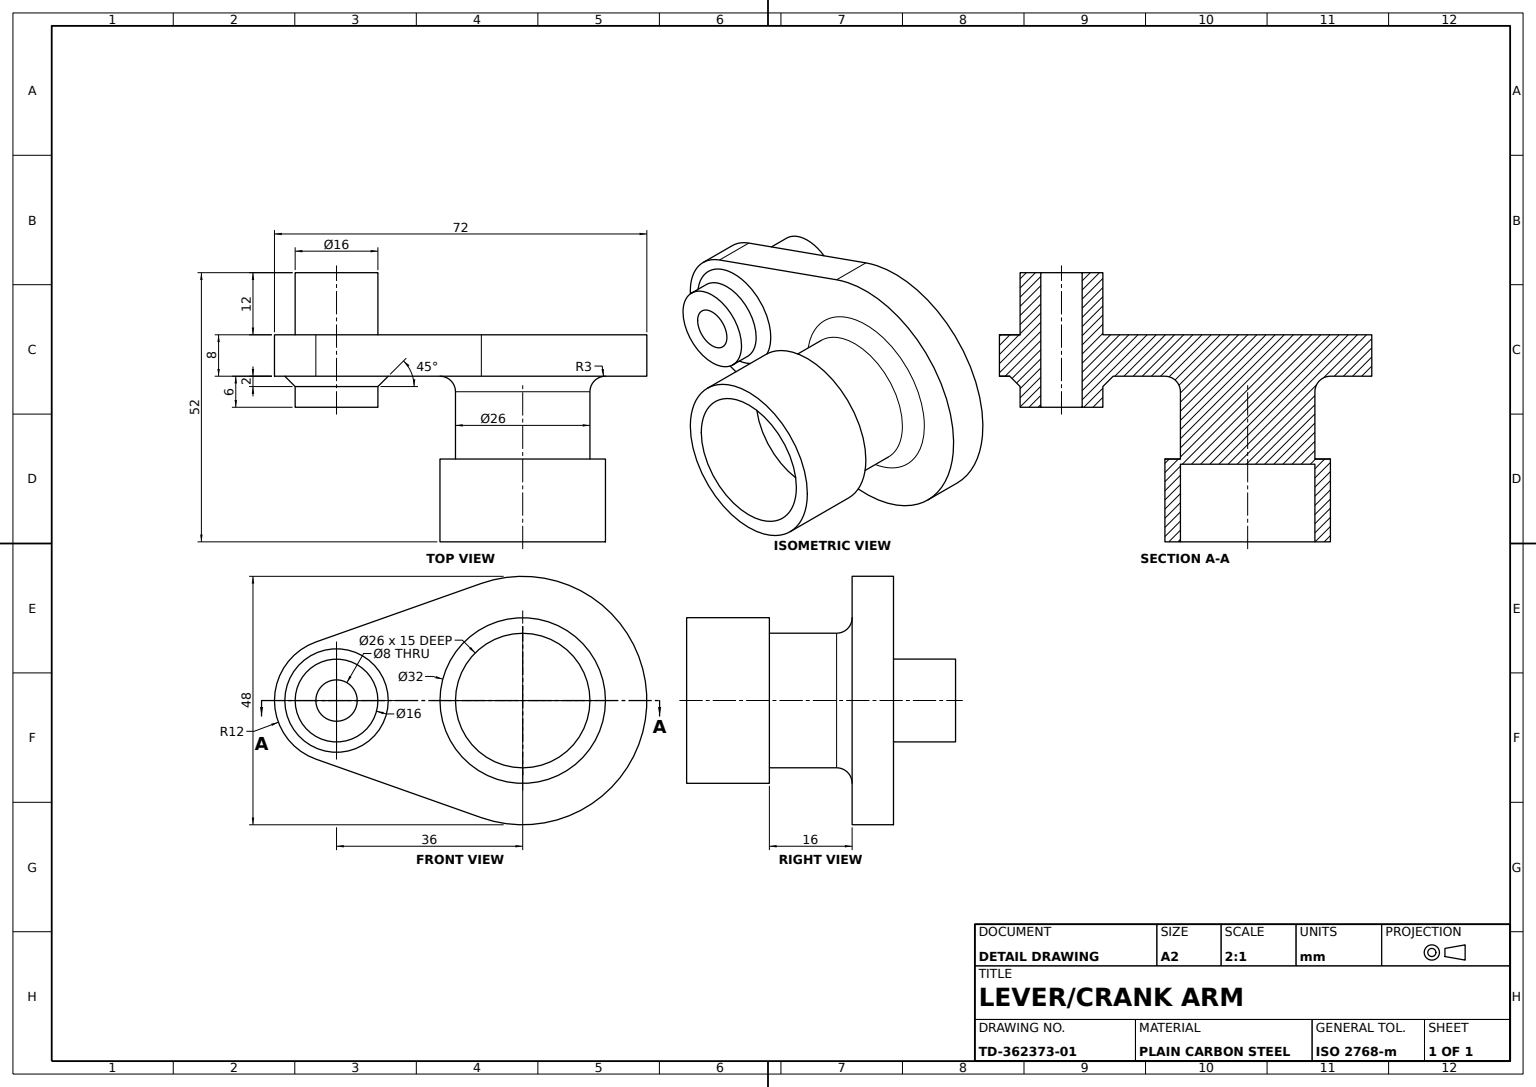
from build123d import *

# Parameters (mm, degrees)
OVAL_PLATE_DEPTH           = 8
PIN_BOSS_SKETCH_R          = 8
PIN_BOSS_DEPTH             = 6
REAR_START                 = 12
REAR_BOSS_SKETCH_R         = 8
REAR_BOSS_DEPTH            = 12
TUBE_NECK_SKETCH_R         = 13
TUBE_NECK_26_DEPTH         = 16
TUBE_BOSS_SKETCH_R         = 16
TUBE_BOSS_32_DEPTH         = 16
TUBE_START                 = -15
TUBE_BORE_SKETCH_R         = 13
TUBE_BORE_26_DEPTH         = 15
TUBE_NECK_ROOT_FILLET_R3_R = 3
PIN_BOSS_CHAMFER_2MM_SIZE  = 2
PIN_HOLE_SKETCH_R          = 4
PIN_THROUGH_HOLE_DEPTH     = 50


with BuildPart() as part:
    # Oval Plate Sketch → Oval Plate (new body)
    with BuildSketch(Plane.XY):
        with BuildLine():
            Line((-40, 11.313708499), (-8, 22.627416998))
            ThreePointArc((-8, 22.627416998), (24, 0), (-8, -22.627416998))
            Line((-8, -22.627416998), (-40, -11.313708499))
            ThreePointArc((-40, -11.313708499), (-48, 0), (-40, 11.313708499))
        make_face()
    extrude(amount=OVAL_PLATE_DEPTH)

    # Pin Boss Sketch → Pin Boss (add)
    with BuildSketch(Plane.XY.offset(8)):
        with Locations((-36, 0)):
            Circle(PIN_BOSS_SKETCH_R)
    extrude(amount=PIN_BOSS_DEPTH)

    # Rear Boss Sketch → Rear Boss (add)
    with BuildSketch(Plane(origin=(0, 0, 0), x_dir=(-1, 0, 0), z_dir=(0, 0, -1)).offset(REAR_START)):
        with Locations(Location((36, 0, 0), (0, 0, 180))):
            Circle(REAR_BOSS_SKETCH_R)
    extrude(amount=-REAR_BOSS_DEPTH)

    # Tube Neck Sketch → Tube Neck Ø26 (add)
    with BuildSketch(Plane.XY.offset(8)):
        Circle(TUBE_NECK_SKETCH_R)
    extrude(amount=TUBE_NECK_26_DEPTH)

    # Tube Boss Sketch → Tube Boss Ø32 (add)
    with BuildSketch(Plane.XY.offset(24)):
        Circle(TUBE_BOSS_SKETCH_R)
    extrude(amount=TUBE_BOSS_32_DEPTH)

    # Tube Bore Sketch → Tube Bore Ø26 (cut)
    with BuildSketch(Plane.XY.offset(40).offset(TUBE_START)):
        Circle(TUBE_BORE_SKETCH_R)
    extrude(amount=TUBE_BORE_26_DEPTH, mode=Mode.SUBTRACT)

    # Tube Neck Root Fillet R3
    tube_neck_root_fillet_r3_edges = [part.edges().sort_by_distance(p)[0] for p in [
        (-13, 0, 8),
    ]]
    fillet(tube_neck_root_fillet_r3_edges, radius=TUBE_NECK_ROOT_FILLET_R3_R)

    # Pin Boss Chamfer 2mm
    pin_boss_chamfer_2mm_edges = [part.edges().sort_by_distance(p)[0] for p in [
        (-44, 0, 8),
    ]]
    chamfer(pin_boss_chamfer_2mm_edges, length=PIN_BOSS_CHAMFER_2MM_SIZE)

    # Pin Hole Sketch → Pin Through Hole (cut)
    with BuildSketch(Plane.XY.offset(14)):
        with Locations((-36, 0)):
            Circle(PIN_HOLE_SKETCH_R)
    extrude(amount=-PIN_THROUGH_HOLE_DEPTH, mode=Mode.SUBTRACT)


solid = part.part
